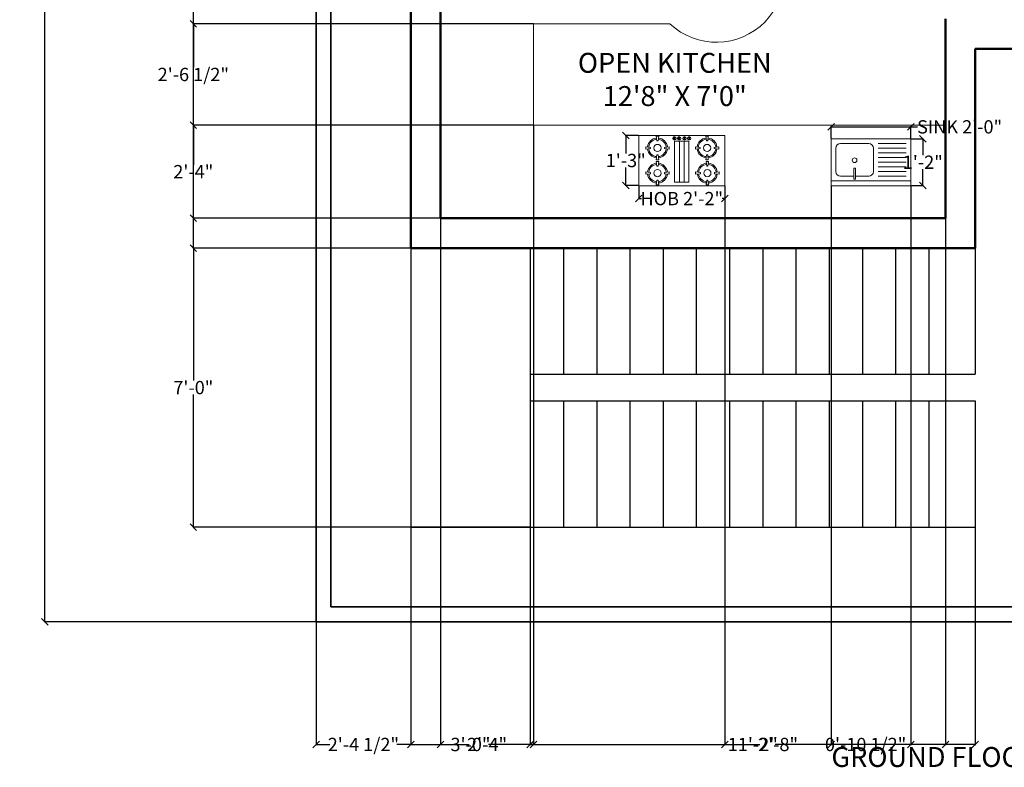
# Model space of a CAD drawing. Units: inches. Extents: x -317284 to 524, y -2236 to 1075.
# Tile 2 of 6: x -24 to 273, y 371 to 596. Entities that reach past the tile are written whole.
import ezdxf

# ---------------------------------------------------------------- set-up
doc = ezdxf.new("R2010")
doc.units = ezdxf.units.IN
doc.header["$MEASUREMENT"] = 0
for name, color, linetype, lineweight in [('A-ANNO-DIMS', 2, 'Continuous', 18), ('A-ANNO-TEXT', 7, 'Continuous', 25), ('A-AREA-IDEN', 7, 'Continuous', 18), ('A-EQPM', 9, 'Continuous', 18), ('A-FLOR-CASE', 8, 'Continuous', 20), ('A-FLOR-FIXT', 9, 'Continuous', 18), ('A-FLOR-STRS', 7, 'Continuous', 25), ('A-WALL', 7, 'Continuous', 50), ('C-PROP', 3, 'Continuous', 35), ('C-SITE-PVMT', 8, 'Continuous', 18)]:
    doc.layers.add(name, color=color, linetype=linetype, lineweight=lineweight)
doc.styles.get("Standard").update_dxf_attribs({"font": 'arial.ttf'})
doc.dimstyles.get("Standard").update_dxf_attribs({"dimtxt": 4, "dimasz": 2, "dimexe": 0.18, "dimexo": 0.0625, "dimgap": 0.09, "dimtad": 0, "dimtih": 1, "dimtoh": 1, "dimdec": 0, "dimzin": 0, "dimdsep": 46, "dimlunit": 4, "dimtxsty": 'Standard', "dimblk": 'OBLIQUE', "dimcen": 0.09, "dimadec": 0, "dimazin": 0, "dimtfac": 1, "dimtdec": 0, "dimtofl": 0, "dimtmove": 0, "dimatfit": 3, "dimldrblk": 'OBLIQUE', "dimfxl": 1, "dimtolj": 1, "dimtzin": 0, "dimarcsym": 0})

# ---------------------------------------------------------------- blocks, each defined once
blk = doc.blocks.new('A$C57CF26DA')
for p, q in [((0, 0), (0, 420)), ((720, 420), (0, 420)), ((166.9, 413), (146.9, 413)), ((146.9, 413), (151.9, 373)), ((161.9, 373), (166.9, 413)), ((583.6, 413), (563.6, 413)), ((563.6, 413), (568.6, 373)), ((578.6, 373), (583.6, 413)), ((720, 0), (720, 420)), ((151.9, 373), (161.9, 373)), ((300, 390.9), (300, 49.1)), ((300, 390.9), (420, 390.9)), ((340, 390.9), (340, 49.1)), ((380, 390.9), (380, 49.1)), ((420, 390.9), (420, 49.1)), ((568.6, 373), (578.6, 373)), ((98.9, 320), (58.9, 325)), ((58.9, 325), (58.9, 305)), ((58.9, 305), (98.9, 310)), ((98.9, 310), (98.9, 320)), ((151.9, 257), (146.9, 217)), ((161.9, 257), (151.9, 257)), ((166.9, 217), (161.9, 257)), ((254.8, 325), (214.8, 320)), ((214.8, 320), (214.8, 310)), ((214.8, 310), (254.8, 305)), ((254.8, 305), (254.8, 325)), ((515.6, 320), (475.6, 325)), ((475.6, 325), (475.6, 305)), ((475.6, 305), (515.6, 310)), ((515.6, 310), (515.6, 320)), ((568.6, 257), (563.6, 217)), ((578.6, 257), (568.6, 257)), ((583.6, 217), (578.6, 257)), ((671.6, 325), (631.6, 320)), ((631.6, 320), (631.6, 310)), ((631.6, 310), (671.6, 305)), ((671.6, 305), (671.6, 325)), ((146.9, 217), (166.9, 217)), ((166.9, 203), (146.9, 203)), ((146.9, 203), (151.9, 163)), ((161.9, 163), (166.9, 203)), ((581.1, 203), (561.1, 203)), ((561.1, 203), (566.1, 163)), ((563.6, 217), (583.6, 217)), ((576.1, 163), (581.1, 203)), ((98.9, 110), (58.9, 115)), ((58.9, 115), (58.9, 95)), ((58.9, 95), (98.9, 100)), ((98.9, 100), (98.9, 110)), ((151.9, 163), (161.9, 163)), ((254.8, 115), (214.8, 110)), ((214.8, 110), (214.8, 100)), ((214.8, 100), (254.8, 95)), ((254.8, 95), (254.8, 115)), ((513.1, 110), (473.1, 115)), ((473.1, 115), (473.1, 95)), ((473.1, 95), (513.1, 100)), ((513.1, 100), (513.1, 110)), ((566.1, 163), (576.1, 163)), ((669, 115), (629, 110)), ((629, 110), (629, 100)), ((629, 100), (669, 95)), ((669, 95), (669, 115)), ((151.9, 47), (146.9, 7)), ((146.9, 7), (166.9, 7)), ((161.9, 47), (151.9, 47)), ((166.9, 7), (161.9, 47)), ((301.5, 38.7), (294.7, 38.7)), ((294.7, 38.7), (294.7, 11.3)), ((294.7, 11.3), (301.5, 11.3)), ((420, 49.1), (300, 49.1)), ((301.5, 11.3), (301.5, 38.7)), ((340.5, 38.7), (333.7, 38.7)), ((333.7, 38.7), (333.7, 11.3)), ((333.7, 11.3), (340.5, 11.3)), ((340.5, 11.3), (340.5, 38.7)), ((379.7, 11.3), (379.7, 38.7)), ((379.7, 38.7), (386.5, 38.7)), ((386.5, 11.3), (379.7, 11.3)), ((386.5, 38.7), (386.5, 11.3)), ((418.7, 11.3), (418.7, 38.7)), ((418.7, 38.7), (425.5, 38.7)), ((425.5, 11.3), (418.7, 11.3)), ((425.5, 38.7), (425.5, 11.3)), ((566.1, 47), (561.1, 7)), ((561.1, 7), (581.1, 7)), ((576.1, 47), (566.1, 47)), ((581.1, 7), (576.1, 47)), ((720, 0), (0, 0))]:
    blk.add_line(p, q)
for centre in [(156.9, 315), (573.6, 315), (156.9, 105), (571.1, 105)]:
    blk.add_circle(centre, 30)
for centre, radius, start, end in [((156.9, 315), 83, 95.58493, 174.41507), ((156.9, 315), 73, 95.37384, 174.62616), ((156.9, 315), 73, 5.37384, 84.62616), ((156.9, 315), 83, 5.58493, 84.41507), ((573.6, 315), 83, 95.58493, 174.41507), ((573.6, 315), 73, 95.37384, 174.62616), ((573.6, 315), 73, 5.37384, 84.62616), ((573.6, 315), 83, 5.58493, 84.41507), ((156.9, 315), 83, 185.58493, 264.41507), ((156.9, 315), 73, 185.37384, 264.62616), ((156.9, 315), 73, 275.37384, 354.62616), ((156.9, 315), 83, 275.58493, 354.41507), ((573.6, 315), 83, 185.58493, 264.41507), ((573.6, 315), 73, 185.37384, 264.62616), ((573.6, 315), 73, 275.37384, 354.62616), ((573.6, 315), 83, 275.58493, 354.41507), ((156.9, 105), 83, 95.58493, 174.41507), ((156.9, 105), 73, 95.37384, 174.62616), ((156.9, 105), 73, 5.37384, 84.62616), ((156.9, 105), 83, 5.58493, 84.41507), ((571.1, 105), 83, 95.58493, 174.41507), ((571.1, 105), 73, 95.37384, 174.62616), ((571.1, 105), 73, 5.37384, 84.62616), ((571.1, 105), 83, 5.58493, 84.41507), ((156.9, 105), 83, 185.58493, 264.41507), ((156.9, 105), 73, 185.37384, 264.62616), ((156.9, 105), 73, 275.37384, 354.62616), ((156.9, 105), 83, 275.58493, 354.41507), ((571.1, 105), 83, 185.58493, 264.41507), ((571.1, 105), 73, 185.37384, 264.62616), ((571.1, 105), 73, 275.37384, 354.62616), ((571.1, 105), 83, 275.58493, 354.41507), ((298.1, 25), 13.7, 104.47751, 255.52249), ((298.1, 25), 13.7, 284.47751, 75.52249), ((337.1, 25), 13.7, 104.47751, 255.52249), ((337.1, 25), 13.7, 284.47751, 75.52249), ((383.1, 25), 13.7, 104.47751, 255.52249), ((383.1, 25), 13.7, 284.47751, 75.52249), ((422.1, 25), 13.7, 104.47751, 255.52249), ((422.1, 25), 13.7, 284.47751, 75.52249)]:
    blk.add_arc(centre, radius, start, end)
blk = doc.blocks.new('A$C3404121D')
for p, q in [((0, 0), (0, 500)), ((0, 500), (850, 500)), ((0, 450), (850, 450)), ((240, 431), (240, 425)), ((260, 431), (240, 431)), ((240, 425), (240, 315)), ((260, 431), (260, 315)), ((850, 500), (850, 0)), ((50, 100), (50, 350)), ((100, 400), (240, 400)), ((240, 315), (260, 315)), ((260, 400), (400, 400)), ((450, 100), (450, 350)), ((502, 400), (801, 400)), ((502, 350), (801, 350)), ((502, 300), (801, 300)), ((502, 250), (801, 250)), ((502, 200), (801, 200)), ((502, 150), (801, 150)), ((850, 0), (0, 0)), ((400, 50), (100, 50)), ((502, 100), (801, 100)), ((801, 50), (502, 50))]:
    blk.add_line(p, q)
blk.add_circle((250, 228), 25)
for centre, start, end in [((100, 350), 90, 180), ((400, 350), 0, 90), ((100, 100), 180, 270), ((400, 100), 270, 0)]:
    blk.add_arc(centre, 50, start, end)
blk = doc.blocks.new('_Oblique')
at = {"color": 0, "linetype": 'ByBlock', "lineweight": -2}
blk.add_line((-0.5, -0.5), (0.5, 0.5), dxfattribs=at)
blk = doc.blocks.new('*D15')
at = {"layer": 'A-ANNO-DIMS', "color": 0, "lineweight": -2, "transparency": 16777216}
for p, q in [((65.66, 1034.38), (-16.14, 1034.38)), ((-15.96, 1034.38), (-15.96, 726.59)), ((-15.96, 414.53), (-15.96, 722.32)), ((65.66, 414.53), (-16.14, 414.53))]:
    blk.add_line(p, q, dxfattribs=at)
at = {"layer": 'Defpoints', "color": 0, "transparency": 16777216}
for p in [(-15.96, 1034.38), (65.73, 1034.38), (65.73, 414.53)]:
    blk.add_point(p, dxfattribs=at)
at = {"layer": 'A-ANNO-DIMS', "color": 0, "lineweight": -2, "transparency": 16777216, "xscale": 2, "yscale": 2, "zscale": 2}
for p, rotation in [((-15.96, 1034.38), 90), ((-15.96, 414.53), 270)]:
    blk.add_blockref('_Oblique', p, dxfattribs=dict(at, rotation=rotation))
at = {"layer": 'A-ANNO-DIMS', "color": 0, "transparency": 16777216, "insert": (-15.96, 724.45), "char_height": 4, "attachment_point": 5}
blk.add_mtext('\\A1;51\'-8"', dxfattribs=at)
blk = doc.blocks.new('*D25')
at = {"layer": 'A-ANNO-DIMS', "color": 0, "lineweight": -2, "transparency": 16777216}
for p, q in [((162.87, 545.75), (162.87, 541.74)), ((188.84, 545.75), (188.84, 541.74)), ((162.87, 541.92), (163.72, 541.92)), ((188.84, 541.92), (187.98, 541.92))]:
    blk.add_line(p, q, dxfattribs=at)
at = {"layer": 'Defpoints', "color": 0, "transparency": 16777216}
for p in [(162.87, 545.82), (188.84, 545.82), (188.84, 541.92)]:
    blk.add_point(p, dxfattribs=at)
at = {"layer": 'A-ANNO-DIMS', "color": 0, "lineweight": -2, "transparency": 16777216, "xscale": 2, "yscale": 2, "zscale": 2, "rotation": 180}
blk.add_blockref('_Oblique', (162.87, 541.92), dxfattribs=at)
at = {"layer": 'A-ANNO-DIMS', "color": 0, "lineweight": -2, "transparency": 16777216, "xscale": 2, "yscale": 2, "zscale": 2}
blk.add_blockref('_Oblique', (188.84, 541.92), dxfattribs=at)
at = {"layer": 'A-ANNO-DIMS', "color": 0, "transparency": 16777216, "insert": (175.85, 541.92), "char_height": 4, "attachment_point": 5}
blk.add_mtext('\\A1;HOB 2\'-2"', dxfattribs=at)
blk = doc.blocks.new('*D26')
at = {"layer": 'A-ANNO-DIMS', "color": 0, "lineweight": -2, "transparency": 16777216}
for p, q in [((162.81, 560.96), (158.79, 560.96)), ((158.97, 560.96), (158.97, 555.52)), ((158.97, 545.82), (158.97, 551.26)), ((162.81, 545.82), (158.79, 545.82))]:
    blk.add_line(p, q, dxfattribs=at)
at = {"layer": 'Defpoints', "color": 0, "transparency": 16777216}
for p in [(162.87, 560.96), (158.97, 545.82), (162.87, 545.82)]:
    blk.add_point(p, dxfattribs=at)
at = {"layer": 'A-ANNO-DIMS', "color": 0, "lineweight": -2, "transparency": 16777216, "xscale": 2, "yscale": 2, "zscale": 2}
for p, rotation in [((158.97, 560.96), 90), ((158.97, 545.82), 270)]:
    blk.add_blockref('_Oblique', p, dxfattribs=dict(at, rotation=rotation))
at = {"layer": 'A-ANNO-DIMS', "color": 0, "transparency": 16777216, "insert": (158.97, 553.39), "char_height": 4, "attachment_point": 5}
blk.add_mtext('\\A1;1\'-3"', dxfattribs=at)
blk = doc.blocks.new('*D31')
at = {"layer": 'A-ANNO-DIMS', "color": 0, "lineweight": -2, "transparency": 16777216}
for p, q in [((220.84, 559.99), (220.84, 563.7)), ((220.84, 563.52), (244.82, 563.52)), ((244.82, 559.99), (244.82, 563.7)), ((244.82, 563.52), (246.82, 563.52))]:
    blk.add_line(p, q, dxfattribs=at)
at = {"layer": 'Defpoints', "color": 0, "transparency": 16777216}
for p in [(244.82, 563.52), (220.84, 559.92), (244.82, 559.92)]:
    blk.add_point(p, dxfattribs=at)
at = {"layer": 'A-ANNO-DIMS', "color": 0, "lineweight": -2, "transparency": 16777216, "xscale": 2, "yscale": 2, "zscale": 2, "rotation": 180}
blk.add_blockref('_Oblique', (220.84, 563.52), dxfattribs=at)
at = {"layer": 'A-ANNO-DIMS', "color": 0, "lineweight": -2, "transparency": 16777216, "xscale": 2, "yscale": 2, "zscale": 2}
blk.add_blockref('_Oblique', (244.82, 563.52), dxfattribs=at)
at = {"layer": 'A-ANNO-DIMS', "color": 0, "transparency": 16777216, "insert": (259.51, 563.52), "char_height": 4, "attachment_point": 5}
blk.add_mtext('\\A1;SINK 2\'-0"', dxfattribs=at)
blk = doc.blocks.new('*D32')
at = {"layer": 'A-ANNO-DIMS', "color": 0, "lineweight": -2, "transparency": 16777216}
for p, q in [((244.88, 559.92), (248.6, 559.92)), ((248.42, 559.92), (248.42, 554.97)), ((248.42, 545.82), (248.42, 550.77)), ((244.88, 545.82), (248.6, 545.82))]:
    blk.add_line(p, q, dxfattribs=at)
at = {"layer": 'Defpoints', "color": 0, "transparency": 16777216}
for p in [(244.82, 559.92), (244.82, 545.82), (248.42, 545.82)]:
    blk.add_point(p, dxfattribs=at)
at = {"layer": 'A-ANNO-DIMS', "color": 0, "lineweight": -2, "transparency": 16777216, "xscale": 2, "yscale": 2, "zscale": 2}
for p, rotation in [((248.42, 559.92), 90), ((248.42, 545.82), 270)]:
    blk.add_blockref('_Oblique', p, dxfattribs=dict(at, rotation=rotation))
at = {"layer": 'A-ANNO-DIMS', "color": 0, "transparency": 16777216, "insert": (248.42, 552.87), "char_height": 4, "attachment_point": 5}
blk.add_mtext('\\A1;1\'-2"', dxfattribs=at)
blk = doc.blocks.new('*D34')
at = {"layer": 'A-ANNO-DIMS', "color": 0, "lineweight": -2, "transparency": 16777216}
for p, q in [((118.16, 748.38), (28.6, 748.38)), ((28.78, 748.38), (28.78, 639.86)), ((28.78, 527.03), (28.78, 635.55)), ((94.16, 527.03), (28.6, 527.03))]:
    blk.add_line(p, q, dxfattribs=at)
at = {"layer": 'Defpoints', "color": 0, "transparency": 16777216}
for p in [(118.23, 748.38), (28.78, 527.03), (94.23, 527.03)]:
    blk.add_point(p, dxfattribs=at)
at = {"layer": 'A-ANNO-DIMS', "color": 0, "lineweight": -2, "transparency": 16777216, "xscale": 2, "yscale": 2, "zscale": 2}
for p, rotation in [((28.78, 748.38), 90), ((28.78, 527.03), 270)]:
    blk.add_blockref('_Oblique', p, dxfattribs=dict(at, rotation=rotation))
at = {"layer": 'A-ANNO-DIMS', "color": 0, "transparency": 16777216, "insert": (28.78, 637.7), "char_height": 4, "attachment_point": 5}
blk.add_mtext('\\A1;18\'-5 1/2"', dxfattribs=at)
blk = doc.blocks.new('*D35')
at = {"layer": 'A-ANNO-DIMS', "color": 0, "lineweight": -2, "transparency": 16777216}
for p, q in [((94.23, 442.97), (94.23, 377.4)), ((65.73, 414.47), (65.73, 377.4)), ((65.73, 377.58), (69.88, 377.58)), ((94.23, 377.58), (90.08, 377.58))]:
    blk.add_line(p, q, dxfattribs=at)
at = {"layer": 'Defpoints', "color": 0, "transparency": 16777216}
for p in [(94.23, 443.03), (65.73, 414.53), (94.23, 377.58)]:
    blk.add_point(p, dxfattribs=at)
at = {"layer": 'A-ANNO-DIMS', "color": 0, "lineweight": -2, "transparency": 16777216, "xscale": 2, "yscale": 2, "zscale": 2, "rotation": 180}
blk.add_blockref('_Oblique', (65.73, 377.58), dxfattribs=at)
at = {"layer": 'A-ANNO-DIMS', "color": 0, "lineweight": -2, "transparency": 16777216, "xscale": 2, "yscale": 2, "zscale": 2}
blk.add_blockref('_Oblique', (94.23, 377.58), dxfattribs=at)
at = {"layer": 'A-ANNO-DIMS', "color": 0, "transparency": 16777216, "insert": (79.98, 377.58), "char_height": 4, "attachment_point": 5}
blk.add_mtext('\\A1;2\'-4 1/2"', dxfattribs=at)
blk = doc.blocks.new('*D43')
at = {"layer": 'A-ANNO-DIMS', "color": 0, "lineweight": -2, "transparency": 16777216}
for p, q in [((130.16, 527.03), (28.6, 527.03)), ((28.78, 527.03), (28.78, 487.16)), ((28.78, 443.03), (28.78, 482.9)), ((130.16, 443.03), (28.6, 443.03))]:
    blk.add_line(p, q, dxfattribs=at)
at = {"layer": 'Defpoints', "color": 0, "transparency": 16777216}
for p in [(28.78, 527.03), (130.23, 527.03), (130.23, 443.03)]:
    blk.add_point(p, dxfattribs=at)
at = {"layer": 'A-ANNO-DIMS', "color": 0, "lineweight": -2, "transparency": 16777216, "xscale": 2, "yscale": 2, "zscale": 2}
for p, rotation in [((28.78, 527.03), 90), ((28.78, 443.03), 270)]:
    blk.add_blockref('_Oblique', p, dxfattribs=dict(at, rotation=rotation))
at = {"layer": 'A-ANNO-DIMS', "color": 0, "transparency": 16777216, "insert": (28.78, 485.03), "char_height": 4, "attachment_point": 5}
blk.add_mtext('\\A1;7\'-0"', dxfattribs=at)
blk = doc.blocks.new('*D44')
at = {"layer": 'A-ANNO-DIMS', "color": 0, "lineweight": -2, "transparency": 16777216}
for p, q in [((130.23, 442.97), (130.23, 377.4)), ((264.23, 442.97), (264.23, 377.4)), ((130.23, 377.58), (190.45, 377.58)), ((264.23, 377.58), (204, 377.58))]:
    blk.add_line(p, q, dxfattribs=at)
at = {"layer": 'Defpoints', "color": 0, "transparency": 16777216}
for p in [(130.23, 443.03), (264.23, 443.03), (264.23, 377.58)]:
    blk.add_point(p, dxfattribs=at)
at = {"layer": 'A-ANNO-DIMS', "color": 0, "lineweight": -2, "transparency": 16777216, "xscale": 2, "yscale": 2, "zscale": 2, "rotation": 180}
blk.add_blockref('_Oblique', (130.23, 377.58), dxfattribs=at)
at = {"layer": 'A-ANNO-DIMS', "color": 0, "lineweight": -2, "transparency": 16777216, "xscale": 2, "yscale": 2, "zscale": 2}
blk.add_blockref('_Oblique', (264.23, 377.58), dxfattribs=at)
at = {"layer": 'A-ANNO-DIMS', "color": 0, "transparency": 16777216, "insert": (197.23, 377.58), "char_height": 4, "attachment_point": 5}
blk.add_mtext('\\A1;11\'-2"', dxfattribs=at)
blk = doc.blocks.new('*D45')
at = {"layer": 'A-ANNO-DIMS', "color": 0, "lineweight": -2, "transparency": 16777216}
for p, q in [((94.23, 442.97), (94.23, 377.4)), ((130.23, 442.97), (130.23, 377.4)), ((94.23, 377.58), (106.82, 377.58)), ((130.23, 377.58), (117.63, 377.58))]:
    blk.add_line(p, q, dxfattribs=at)
at = {"layer": 'Defpoints', "color": 0, "transparency": 16777216}
for p in [(94.23, 443.03), (130.23, 443.03), (130.23, 377.58)]:
    blk.add_point(p, dxfattribs=at)
at = {"layer": 'A-ANNO-DIMS', "color": 0, "lineweight": -2, "transparency": 16777216, "xscale": 2, "yscale": 2, "zscale": 2, "rotation": 180}
blk.add_blockref('_Oblique', (94.23, 377.58), dxfattribs=at)
at = {"layer": 'A-ANNO-DIMS', "color": 0, "lineweight": -2, "transparency": 16777216, "xscale": 2, "yscale": 2, "zscale": 2}
blk.add_blockref('_Oblique', (130.23, 377.58), dxfattribs=at)
at = {"layer": 'A-ANNO-DIMS', "color": 0, "transparency": 16777216, "insert": (112.23, 377.58), "char_height": 4, "attachment_point": 5}
blk.add_mtext('\\A1;3\'-0"', dxfattribs=at)
blk = doc.blocks.new('*D47')
at = {"layer": 'A-ANNO-DIMS', "color": 0, "lineweight": -2, "transparency": 16777216}
for p, q in [((131.23, 563.97), (131.23, 377.4)), ((103.23, 535.97), (103.23, 377.4)), ((103.23, 377.58), (111.79, 377.58)), ((131.23, 377.58), (122.67, 377.58))]:
    blk.add_line(p, q, dxfattribs=at)
at = {"layer": 'Defpoints', "color": 0, "transparency": 16777216}
for p in [(131.23, 564.03), (103.23, 536.03), (131.23, 377.58)]:
    blk.add_point(p, dxfattribs=at)
at = {"layer": 'A-ANNO-DIMS', "color": 0, "lineweight": -2, "transparency": 16777216, "xscale": 2, "yscale": 2, "zscale": 2, "rotation": 180}
blk.add_blockref('_Oblique', (103.23, 377.58), dxfattribs=at)
at = {"layer": 'A-ANNO-DIMS', "color": 0, "lineweight": -2, "transparency": 16777216, "xscale": 2, "yscale": 2, "zscale": 2}
blk.add_blockref('_Oblique', (131.23, 377.58), dxfattribs=at)
at = {"layer": 'A-ANNO-DIMS', "color": 0, "transparency": 16777216, "insert": (117.23, 377.58), "char_height": 4, "attachment_point": 5}
blk.add_mtext('\\A1;2\'-4"', dxfattribs=at)
blk = doc.blocks.new('*D48')
at = {"layer": 'A-ANNO-DIMS', "color": 0, "lineweight": -2, "transparency": 16777216}
for p, q in [((131.16, 564.03), (28.6, 564.03)), ((28.78, 564.03), (28.78, 552.13)), ((28.78, 536.03), (28.78, 547.93)), ((103.16, 536.03), (28.6, 536.03))]:
    blk.add_line(p, q, dxfattribs=at)
at = {"layer": 'Defpoints', "color": 0, "transparency": 16777216}
for p in [(28.78, 564.03), (131.23, 564.03), (103.23, 536.03)]:
    blk.add_point(p, dxfattribs=at)
at = {"layer": 'A-ANNO-DIMS', "color": 0, "lineweight": -2, "transparency": 16777216, "xscale": 2, "yscale": 2, "zscale": 2}
for p, rotation in [((28.78, 564.03), 90), ((28.78, 536.03), 270)]:
    blk.add_blockref('_Oblique', p, dxfattribs=dict(at, rotation=rotation))
at = {"layer": 'A-ANNO-DIMS', "color": 0, "transparency": 16777216, "insert": (28.78, 550.03), "char_height": 4, "attachment_point": 5}
blk.add_mtext('\\A1;2\'-4"', dxfattribs=at)
blk = doc.blocks.new('*D49')
at = {"layer": 'A-ANNO-DIMS', "color": 0, "lineweight": -2, "transparency": 16777216}
for p, q in [((131.16, 594.53), (28.6, 594.53)), ((28.78, 594.53), (28.78, 581.44)), ((28.78, 564.03), (28.78, 577.12)), ((131.16, 564.03), (28.6, 564.03))]:
    blk.add_line(p, q, dxfattribs=at)
at = {"layer": 'Defpoints', "color": 0, "transparency": 16777216}
for p in [(131.23, 594.53), (28.78, 564.03), (131.23, 564.03)]:
    blk.add_point(p, dxfattribs=at)
at = {"layer": 'A-ANNO-DIMS', "color": 0, "lineweight": -2, "transparency": 16777216, "xscale": 2, "yscale": 2, "zscale": 2}
for p, rotation in [((28.78, 594.53), 90), ((28.78, 564.03), 270)]:
    blk.add_blockref('_Oblique', p, dxfattribs=dict(at, rotation=rotation))
at = {"layer": 'A-ANNO-DIMS', "color": 0, "transparency": 16777216, "insert": (28.78, 579.28), "char_height": 4, "attachment_point": 5}
blk.add_mtext('\\A1;2\'-6 1/2"', dxfattribs=at)
blk = doc.blocks.new('*D50')
at = {"layer": 'A-ANNO-DIMS', "color": 0, "lineweight": -2, "transparency": 16777216}
for p, q in [((244.82, 545.75), (244.82, 377.4)), ((255.23, 535.97), (255.23, 377.4)), ((244.82, 377.58), (242.82, 377.58)), ((255.23, 377.58), (244.82, 377.58))]:
    blk.add_line(p, q, dxfattribs=at)
at = {"layer": 'Defpoints', "color": 0, "transparency": 16777216}
for p in [(244.82, 545.82), (255.23, 536.03), (244.82, 377.58)]:
    blk.add_point(p, dxfattribs=at)
at = {"layer": 'A-ANNO-DIMS', "color": 0, "lineweight": -2, "transparency": 16777216, "xscale": 2, "yscale": 2, "zscale": 2, "rotation": 180}
blk.add_blockref('_Oblique', (244.82, 377.58), dxfattribs=at)
at = {"layer": 'A-ANNO-DIMS', "color": 0, "lineweight": -2, "transparency": 16777216, "xscale": 2, "yscale": 2, "zscale": 2}
blk.add_blockref('_Oblique', (255.23, 377.58), dxfattribs=at)
at = {"layer": 'A-ANNO-DIMS', "color": 0, "transparency": 16777216, "insert": (231.2, 377.58), "char_height": 4, "attachment_point": 5}
blk.add_mtext('\\A1;0\'-10 1/2"', dxfattribs=at)
blk = doc.blocks.new('*D51')
at = {"layer": 'A-ANNO-DIMS', "color": 0, "lineweight": -2, "transparency": 16777216}
for p, q in [((188.84, 545.75), (188.84, 377.4)), ((220.84, 545.75), (220.84, 377.4)), ((188.84, 377.58), (199.4, 377.58)), ((220.84, 377.58), (210.28, 377.58))]:
    blk.add_line(p, q, dxfattribs=at)
at = {"layer": 'Defpoints', "color": 0, "transparency": 16777216}
for p in [(188.84, 545.82), (220.84, 545.82), (220.84, 377.58)]:
    blk.add_point(p, dxfattribs=at)
at = {"layer": 'A-ANNO-DIMS', "color": 0, "lineweight": -2, "transparency": 16777216, "xscale": 2, "yscale": 2, "zscale": 2, "rotation": 180}
blk.add_blockref('_Oblique', (188.84, 377.58), dxfattribs=at)
at = {"layer": 'A-ANNO-DIMS', "color": 0, "lineweight": -2, "transparency": 16777216, "xscale": 2, "yscale": 2, "zscale": 2}
blk.add_blockref('_Oblique', (220.84, 377.58), dxfattribs=at)
at = {"layer": 'A-ANNO-DIMS', "color": 0, "transparency": 16777216, "insert": (204.84, 377.58), "char_height": 4, "attachment_point": 5}
blk.add_mtext('\\A1;2\'-8"', dxfattribs=at)

msp = doc.modelspace()

# ---------------------------------------------------------------- linework, layer by layer
at = {"layer": 'A-FLOR-CASE'}
for p, q in [((131.23, 594.53), (172.23, 594.53)), ((131.23, 594.53), (131.23, 564.03)), ((131.23, 564.03), (255.23, 564.03))]:
    msp.add_line(p, q, dxfattribs=at)
msp.add_arc((186.25, 609.53), 20.53, 226.9294, 133.0706, dxfattribs=at)
at = {"layer": 'A-FLOR-STRS'}
for p, q in [((94.23, 527.03), (94.23, 443.03)), ((130.23, 527.03), (130.23, 443.03)), ((140.23, 527.03), (140.23, 489.03)), ((150.23, 527.03), (150.23, 489.03)), ((160.23, 527.03), (160.23, 489.03)), ((170.23, 527.03), (170.23, 489.03)), ((180.23, 527.03), (180.23, 489.03)), ((190.23, 527.03), (190.23, 489.03)), ((200.23, 527.03), (200.23, 489.03)), ((210.23, 527.03), (210.23, 489.03)), ((220.23, 527.03), (220.23, 489.03)), ((230.23, 527.03), (230.23, 489.03)), ((240.23, 527.03), (240.23, 489.03)), ((250.23, 527.03), (250.23, 489.03)), ((264.23, 527.03), (264.23, 489.03)), ((130.23, 489.03), (264.23, 489.03)), ((130.23, 481.03), (264.23, 481.03)), ((140.23, 481.03), (140.23, 443.03)), ((150.23, 481.03), (150.23, 443.03)), ((160.23, 481.03), (160.23, 443.03)), ((170.23, 481.03), (170.23, 443.03)), ((180.23, 481.03), (180.23, 443.03)), ((190.23, 481.03), (190.23, 443.03)), ((200.23, 481.03), (200.23, 443.03)), ((210.23, 481.03), (210.23, 443.03)), ((220.23, 481.03), (220.23, 443.03)), ((230.23, 481.03), (230.23, 443.03)), ((240.23, 481.03), (240.23, 443.03)), ((250.23, 481.03), (250.23, 443.03)), ((264.23, 481.03), (264.23, 443.03)), ((94.23, 443.03), (264.23, 443.03))]:
    msp.add_line(p, q, dxfattribs=at)
at = {"layer": 'A-WALL'}
for p, q in [((94.23, 620.03), (94.23, 536.03)), ((103.23, 620.03), (103.23, 536.03)), ((255.23, 536.03), (255.23, 596.03)), ((264.23, 527.03), (264.23, 587.03)), ((264.23, 587.03), (398.73, 587.03)), ((94.23, 536.03), (94.23, 527.03)), ((103.23, 536.03), (255.23, 536.03)), ((94.23, 527.03), (103.23, 527.03)), ((103.23, 527.03), (255.23, 527.03)), ((255.23, 527.03), (264.23, 527.03))]:
    msp.add_line(p, q, dxfattribs=at)
at = {"layer": 'C-PROP'}
for points in [[(475.23, 1034.38), (475.23, 414.53), (65.73, 414.53), (65.73, 1034.38)], [(470.73, 1029.88), (470.73, 419.03), (70.23, 419.03), (70.23, 1029.88)]]:
    msp.add_lwpolyline(points, close=True, dxfattribs=at)
at = {"layer": 'C-SITE-PVMT'}
msp.add_line((264.23, 443.03), (264.23, 419.03), dxfattribs=at)

# ---------------------------------------------------------------- block references
at = {"layer": 'A-EQPM', "xscale": -0.0360698337762115, "yscale": 0.0360698337762115, "zscale": 0.0360698337762115, "rotation": 180}
msp.add_blockref('A$C57CF26DA', (162.87, 560.96), dxfattribs=at)
at = {"layer": 'A-FLOR-FIXT', "xscale": -0.0282142316244683, "yscale": 0.0282142316244683, "zscale": 0.0282142316244683, "rotation": 180}
msp.add_blockref('A$C3404121D', (220.84, 559.92), dxfattribs=at)

# ---------------------------------------------------------------- texts
at = {"layer": 'A-ANNO-TEXT', "insert": (220.89, 376.82), "char_height": 6, "attachment_point": 1}
msp.add_mtext_dynamic_manual_height_columns('GROUND FLOOR PLAN', width=269.2345, gutter_width=30, heights=[0], dxfattribs=at)
at = {"layer": 'A-AREA-IDEN', "insert": (112.71, 585.79), "char_height": 6, "attachment_point": 1}
msp.add_mtext_dynamic_manual_height_columns('\\pxqc;OPEN KITCHEN\\P12\'8" X 7\'0"', width=122.0512, gutter_width=30, heights=[0], dxfattribs=at)

# ---------------------------------------------------------------- dimensions: what is measured, and where the dimension line sits
at = {"layer": 'A-ANNO-DIMS'}
for base, p1, p2, angle, override, picture, middle in [((-15.96, 1034.38), (65.73, 414.53), (65.73, 1034.38), 90, {"dimclrd": 0, "dimclre": 0, "dimclrt": 0}, '*D15', (-15.96, 724.45)), ((28.7766, 527.0289), (118.2266, 748.3794), (94.2266, 527.0289), 90, {"dimdec": 1, "dimlfac": 1, "dimrnd": 0, "dimzin": 1, "dimdsep": 46, "dimlunit": 4, "dimfrac": 2}, '*D34', (28.7766, 637.7042)), ((28.78, 564.03), (131.23, 594.53), (131.23, 564.03), 90, {"dimdec": 1, "dimlfac": 1, "dimrnd": 0, "dimzin": 1, "dimdsep": 46, "dimlunit": 4, "dimfrac": 2}, '*D49', (28.78, 579.28)), ((28.78, 564.03), (103.23, 536.03), (131.23, 564.03), 90, {"dimdec": 1, "dimlfac": 1, "dimrnd": 0, "dimzin": 1, "dimdsep": 46, "dimlunit": 4, "dimfrac": 2}, '*D48', (28.78, 550.03)), ((158.97, 545.82), (162.87, 560.96), (162.87, 545.82), 270, {"dimdec": 1, "dimlfac": 1, "dimrnd": 0, "dimzin": 1, "dimdsep": 46, "dimlunit": 4, "dimfrac": 2}, '*D26', (158.97, 553.39)), ((248.42, 545.82), (244.82, 559.92), (244.82, 545.82), 270, {"dimdec": 1, "dimlfac": 1, "dimrnd": 0, "dimzin": 1, "dimdsep": 46, "dimlunit": 4, "dimfrac": 2}, '*D32', (248.42, 552.87)), ((28.78, 527.03), (130.23, 443.03), (130.23, 527.03), 90, {"dimdec": 1, "dimlfac": 1, "dimrnd": 0, "dimzin": 1, "dimdsep": 46, "dimlunit": 4, "dimfrac": 2}, '*D43', (28.78, 485.03))]:
    dim = msp.add_linear_dim(base=base, p1=p1, p2=p2, angle=angle, dimstyle='Standard', override=override, dxfattribs=at)
    dim.commit()
    dim.dimension.update_dxf_attribs({"geometry": picture, "text_midpoint": middle})
for base, p1, p2, text, picture, middle in [((244.82, 563.52), (220.84, 559.92), (244.82, 559.92), 'SINK <>', '*D31', (259.51, 563.52)), ((188.84, 541.92), (162.87, 545.82), (188.84, 545.82), 'HOB <>', '*D25', (175.85, 541.92))]:
    dim = msp.add_linear_dim(base=base, p1=p1, p2=p2, text=text, dimstyle='Standard', override={"dimdec": 1, "dimlfac": 1, "dimrnd": 0, "dimzin": 1, "dimdsep": 46, "dimlunit": 4, "dimfrac": 2}, dxfattribs=at)
    dim.commit()
    dim.dimension.update_dxf_attribs({"geometry": picture, "text_midpoint": middle})
for base, p1, p2, picture, middle in [((131.23, 377.58), (103.23, 536.03), (131.23, 564.03), '*D47', (117.23, 377.58)), ((220.84, 377.58), (188.84, 545.82), (220.84, 545.82), '*D51', (204.84, 377.58)), ((244.82, 377.58), (255.23, 536.03), (244.82, 545.82), '*D50', (231.2, 377.58)), ((94.23, 377.58), (65.73, 414.53), (94.23, 443.03), '*D35', (79.98, 377.58)), ((130.23, 377.58), (94.23, 443.03), (130.23, 443.03), '*D45', (112.23, 377.58)), ((264.23, 377.58), (130.23, 443.03), (264.23, 443.03), '*D44', (197.23, 377.58))]:
    dim = msp.add_linear_dim(base=base, p1=p1, p2=p2, dimstyle='Standard', override={"dimdec": 1, "dimlfac": 1, "dimrnd": 0, "dimzin": 1, "dimdsep": 46, "dimlunit": 4, "dimfrac": 2}, dxfattribs=at)
    dim.commit()
    dim.dimension.update_dxf_attribs({"geometry": picture, "text_midpoint": middle})

doc.saveas('drawing.dxf')
